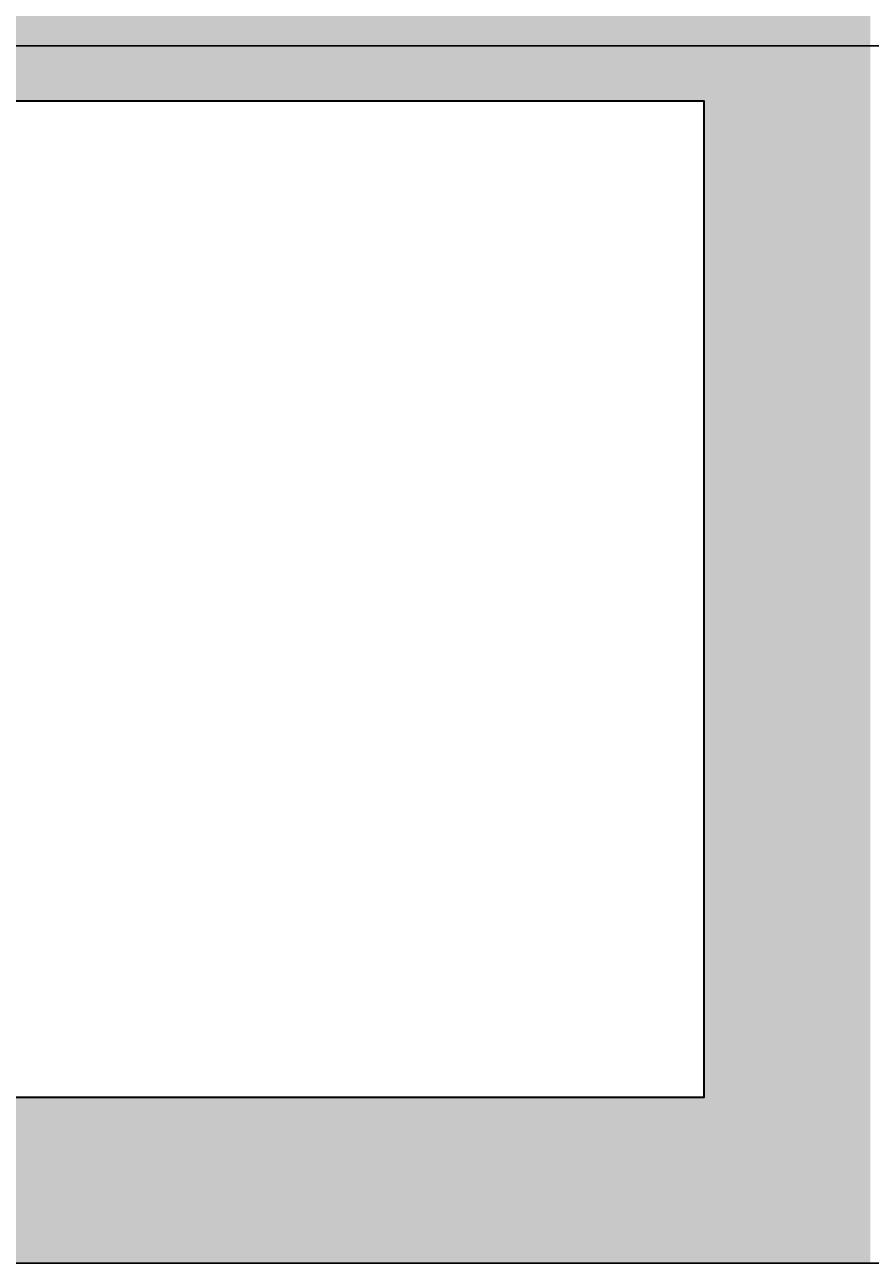
# Model space of a CAD drawing. Units: inches. Extents: x 1998 to 2588, y 1139 to 1977.
# Tile 104 of 134: x 2452 to 2498, y 1523 to 1590. Entities that reach past the tile are written whole.
import ezdxf

# ---------------------------------------------------------------- set-up
doc = ezdxf.new("R2010")
doc.units = ezdxf.units.IN
for name, color, linetype, lineweight in [('A-ANNO-DIMS', 2, 'Continuous', 18), ('A-FLOR-EVTR', 7, 'Continuous', 35), ('A-WALL-PATT', 252, 'Continuous', 13)]:
    doc.layers.add(name, color=color, linetype=linetype, lineweight=lineweight)
doc.styles.get("Standard").update_dxf_attribs({"font": 'arial.ttf'})
doc.dimstyles.get("Standard").update_dxf_attribs({"dimtxt": 0.18, "dimasz": 0.18, "dimexe": 0.18, "dimexo": 0.0625, "dimgap": 0.09, "dimtad": 0, "dimtih": 1, "dimtoh": 1, "dimdec": 4, "dimzin": 0, "dimdsep": 46, "dimtxsty": 'Standard', "dimcen": 0.09, "dimadec": 0, "dimazin": 0, "dimtfac": 1, "dimtdec": 4, "dimtofl": 0, "dimtmove": 0, "dimatfit": 3, "dimfxl": 1, "dimtolj": 1, "dimtzin": 0, "dimarcsym": 0})

# ---------------------------------------------------------------- blocks, each defined once
blk = doc.blocks.new('*D24')
at = {"layer": 'A-ANNO-DIMS', "color": 0, "lineweight": -2, "transparency": 16777216}
for p, q in [((2398.535, 1911.232), (2588.309, 1911.232)), ((2588.129, 1911.052), (2588.129, 1570.164)), ((2588.129, 1228.912), (2588.129, 1569.8)), ((2527.535, 1228.732), (2588.309, 1228.732))]:
    blk.add_line(p, q, dxfattribs=at)
at = {"layer": 'A-ANNO-DIMS', "color": 0, "transparency": 16777216}
for points in [[(2588.099, 1911.052), (2588.159, 1911.052), (2588.129, 1911.232)], [(2588.099, 1228.912), (2588.159, 1228.912), (2588.129, 1228.732)]]:
    blk.add_solid(points, dxfattribs=at)
at = {"layer": 'Defpoints', "color": 0, "transparency": 16777216}
for p in [(2398.473, 1911.232), (2588.129, 1911.232), (2527.473, 1228.732)]:
    blk.add_point(p, dxfattribs=at)
at = {"layer": 'A-ANNO-DIMS', "color": 0, "transparency": 16777216, "insert": (2588.129, 1569.982), "char_height": 0.18, "attachment_point": 5}
blk.add_mtext('\\A1;682.5', dxfattribs=at)
blk = doc.blocks.new('*D42')
at = {"layer": 'A-ANNO-DIMS', "color": 0, "lineweight": -2, "transparency": 16777216}
for p, q in [((2287.535, 1588.732), (2588.309, 1588.732)), ((2588.129, 1588.552), (2588.129, 1555.914)), ((2588.129, 1522.912), (2588.129, 1555.55)), ((2287.535, 1522.732), (2588.309, 1522.732))]:
    blk.add_line(p, q, dxfattribs=at)
at = {"layer": 'A-ANNO-DIMS', "color": 0, "transparency": 16777216}
for points in [[(2588.099, 1588.552), (2588.159, 1588.552), (2588.129, 1588.732)], [(2588.099, 1522.912), (2588.159, 1522.912), (2588.129, 1522.732)]]:
    blk.add_solid(points, dxfattribs=at)
at = {"layer": 'Defpoints', "color": 0, "transparency": 16777216}
for p in [(2287.473, 1588.732), (2588.129, 1588.732), (2287.473, 1522.732)]:
    blk.add_point(p, dxfattribs=at)
at = {"layer": 'A-ANNO-DIMS', "color": 0, "transparency": 16777216, "insert": (2588.129, 1555.732), "char_height": 0.18, "attachment_point": 5}
blk.add_mtext('\\A1;66', dxfattribs=at)

msp = doc.modelspace()

# ---------------------------------------------------------------- hatches: boundary and pattern name
at = {"layer": 'A-WALL-PATT'}
h = msp.add_hatch(color=256, dxfattribs=at)
h.dxf.hatch_style = 1
h.paths.add_polyline_path([(2527.4729, 1362.2324), (2510.9729, 1362.2324), (2510.9729, 1357.7324), (2518.4729, 1357.7324), (2518.4729, 1237.7324), (2503.1458, 1237.7324), (2503.1458, 1228.7324), (2527.4729, 1228.7324)])
h.paths.add_polyline_path([(2490.5682, 1362.2324), (2398.4729, 1362.2324), (2398.4729, 1357.7324), (2490.5682, 1357.7324)])
h.paths.add_polyline_path([(2224.9729, 1264.7324), (2222.9729, 1264.7324), (2222.9729, 1232.4125), (2341.4729, 1232.4125), (2341.4729, 1234.4125), (2224.9729, 1234.4125)])
h.paths.add_polyline_path([(2334.5332, 1273.7324), (2264.7638, 1273.7324), (2264.7638, 1269.5611, -0.043659), (2264.3413, 1264.7324), (2334.5332, 1264.7324)])
h.paths.add_polyline_path([(2236.9551, 1273.7324), (2234.4125, 1273.7324), (2234.4125, 1264.7324), (2236.9551, 1264.7324), (2236.9551, 1269.5611)])
h.paths.add_polyline_path([(2222.9729, 1293.2324), (2096.9729, 1293.2324), (2096.9729, 1345.0966), (2087.9729, 1345.0966), (2087.9729, 1284.2324), (2222.9729, 1284.2324), (2222.9729, 1285.137)])
h.paths.add_polyline_path([(2096.9729, 1458.7927), (2087.9729, 1458.7927), (2087.9729, 1417.7324), (2087.9729, 1413.2324), (2096.9729, 1413.2324), (2096.9729, 1417.7324)])
h.paths.add_polyline_path([(2096.9729, 1413.2324), (2087.9729, 1413.2324), (2087.9729, 1365.5012), (2096.9729, 1365.5012), (2096.9729, 1369.3358)])
h.paths.add_polyline_path([(2186.2943, 1417.7324), (2138.6074, 1417.7324), (2096.9729, 1417.7324), (2096.9729, 1413.2324), (2138.6074, 1413.2324), (2186.2943, 1413.2324)])
h.paths.add_polyline_path([(2181.4729, 1465.7324), (2176.9729, 1465.7324), (2176.9729, 1451.6434), (2181.4729, 1451.6434)])
h.paths.add_polyline_path([(2181.4729, 1422.1664), (2176.9729, 1422.1664), (2176.9729, 1417.7324), (2181.4729, 1417.7324)])
h.paths.add_polyline_path([(2063.9729, 1465.7324), (2087.9729, 1465.7324), (2087.9729, 1470.2324), (2059.4729, 1470.2324), (2059.4729, 1413.2324), (2087.9729, 1413.2324), (2087.9729, 1417.7324), (2063.9729, 1417.7324)])
h.paths.add_polyline_path([(2181.4729, 1755.2324), (2176.9729, 1755.2324), (2176.9729, 1748.6798), (2177.0513, 1748.6798), (2181.4729, 1748.6798)])
h.paths.add_polyline_path([(2227.4729, 1707.2324), (2220.4647, 1707.2324), (2220.4647, 1702.7324), (2222.9729, 1702.7324), (2222.9729, 1604.637), (2227.4729, 1604.637)])
h.paths.add_polyline_path([(2114.9729, 1702.7324), (2105.9729, 1702.7324), (2105.9729, 1628.4781, -0.0318759), (2110.1012, 1628.7416), (2114.9729, 1628.7416)])
h.paths.add_polyline_path([(2345.9729, 1739.3278), (2341.4729, 1739.3278), (2341.4729, 1647.5211), (2345.9729, 1647.5211)])
h.paths.add_polyline_path([(2350.6273, 1641.2324), (2345.9729, 1641.2324), (2345.9729, 1636.7324), (2350.6273, 1636.7324), (2350.6273, 1639.8729)])
h.paths.add_polyline_path([(2501.9729, 1641.2324), (2407.9729, 1641.2324), (2392.5005, 1641.2324), (2392.5005, 1639.8729), (2392.5005, 1636.7324), (2501.9729, 1636.7324)])
h.paths.add_polyline_path([(2510.9729, 1755.2324), (2501.9729, 1755.2324), (2501.9729, 1641.2324), (2510.9729, 1641.2324)])
h.paths.add_polyline_path([(2549.1786, 1641.2324), (2522.3775, 1641.2324), (2522.3775, 1636.7324), (2540.1786, 1636.7324), (2540.1786, 1480.7324), (2522.3775, 1480.7324), (2522.3775, 1476.2324), (2549.1786, 1476.2324)])
h.paths.add_polyline_path([(2498.1786, 1594.7324), (2407.9729, 1594.7324), (2407.9729, 1585.7324), (2416.9729, 1585.7324), (2489.1786, 1585.7324), (2489.1786, 1531.7324), (2416.9729, 1531.7324), (2407.9729, 1531.7324), (2407.9729, 1522.7324), (2498.1786, 1522.7324)])
h.paths.add_polyline_path([(2351.6437, 1480.7324), (2345.9729, 1480.7324), (2345.9729, 1476.2324), (2351.6437, 1476.2324), (2351.6437, 1477.5919)])
h.paths.add_polyline_path([(2501.9729, 1480.7324), (2498.1786, 1480.7324), (2407.9729, 1480.7324), (2393.5168, 1480.7324), (2393.5168, 1477.5919), (2393.5168, 1476.2324), (2501.9729, 1476.2324)])

# ---------------------------------------------------------------- linework, layer by layer
at = {"layer": 'A-FLOR-EVTR'}
msp.add_lwpolyline([(2416.9729, 1531.7324), (2489.1786, 1531.7324), (2489.1786, 1585.7324), (2416.9729, 1585.7324)], dxfattribs=at)

# ---------------------------------------------------------------- dimensions: what is measured, and where the dimension line sits
at = {"layer": 'A-ANNO-DIMS'}
for base, p1, p2, override, picture, middle in [((2588.1286, 1911.2324), (2527.4729, 1228.7324), (2398.4729, 1911.2324), {"dimdec": 1, "dimlfac": 1, "dimrnd": 0, "dimzin": 0, "dimdsep": 46, "dimlunit": 2}, '*D24', (2588.1286, 1569.9824)), ((2588.1286, 1588.7324), (2287.4729, 1522.7324), (2287.4729, 1588.7324), {"dimdec": 0, "dimlfac": 1, "dimrnd": 0, "dimzin": 0, "dimdsep": 46, "dimlunit": 2}, '*D42', (2588.1286, 1555.7324))]:
    dim = msp.add_linear_dim(base=base, p1=p1, p2=p2, angle=90, dimstyle='Standard', override=override, dxfattribs=at)
    dim.commit()
    dim.dimension.update_dxf_attribs({"geometry": picture, "text_midpoint": middle})

doc.saveas('drawing.dxf')
